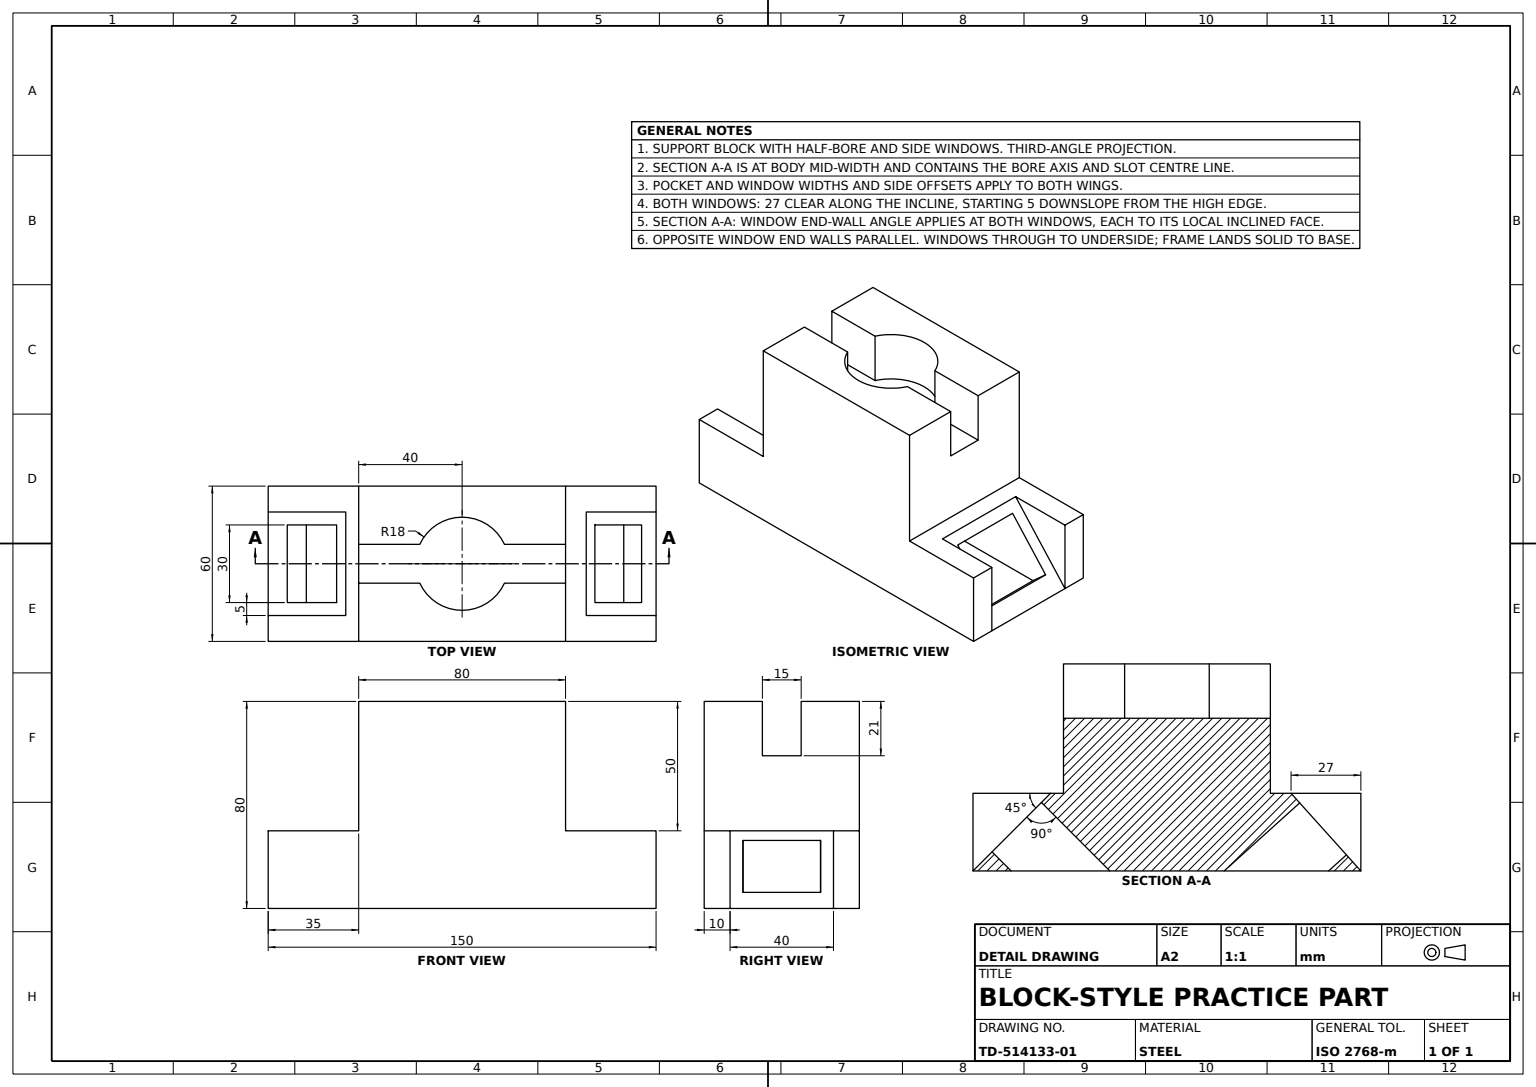
SolidWorks part; units mm, degrees
material "Plain Carbon Steel"
ref_plane "Front Plane" through (0, 0, 0) normal (0, 0, 1) x (1, 0, 0)
ref_plane "Top Plane" through (0, 0, 0) normal (0, 1, 0) x (1, 0, 0)
ref_plane "Right Plane" through (0, 0, 0) normal (1, 0, 0) x (0, 0, -1)
sketch "Base Profile Sketch" plane through (0, 0, 0) normal (0, 0, 1) x (1, 0, 0)
  line L0 (-47.8178, 0) -> (102.1822, 0)
  line L1 (102.1822, 0) -> (102.1822, 30)
  line L2 (102.1822, 30) -> (67.1822, 30)
  line L3 (67.1822, 30) -> (67.1822, 80)
  line L4 (67.1822, 80) -> (-12.8178, 80)
  line L5 (-12.8178, 80) -> (-12.8178, 30)
  line L6 (-12.8178, 30) -> (-47.8178, 30)
  line L7 (-47.8178, 30) -> (-47.8178, 0)
  dimension "D1" = 150
  dimension "D2" = 30
  dimension "D3" = 35
  dimension "D4" = 50
  dimension "D5" = 50
  dimension "D6" = 80
  dimension "D7" = 47.8178
extrude "Base Block" add sketch "Base Profile Sketch" against normal blind 60
sketch "Bore Sketch" plane through (0, 80, 0) normal (0, 1, 0) x (1, 0, 0)
  line L0 (-12.8178, 60) -> (-12.8178, 0) construction
  line L1 (67.1822, 0) -> (-12.8178, 0) construction
  circle A1 centre (27.1822, 30) radius 18
  point P4 (-12.8178, 30)
  dimension "D1" = 18
  dimension "D2" = 40
  dimension "D3" = 30
extrude "Half Bore Cut" cut sketch "Bore Sketch" against normal blind 21
sketch "Top Slot Sketch" plane through (0, 80, 0) normal (0, 1, 0) x (1, 0, 0)
  line L0 (-12.8178, 37.5) -> (-12.8178, 22.5)
  line L1 (67.1822, 37.5) -> (67.1822, 22.5)
  line L3 (-12.8178, 22.5) -> (67.1822, 22.5)
  line L4 (-12.8178, 37.5) -> (67.1822, 37.5)
  dimension "D1" = 15
  dimension "D2" = 80
  dimension "D3" = 12.8178
  dimension "D4" = 22.5
extrude "Top Slot Cut" cut sketch "Top Slot Sketch" against normal blind 21
sketch "Side Pocket A Sketch" plane through (0, 30, 0) normal (0, 1, 0) x (1, 0, 0)
  line L2 (102.1822, 60) -> (102.1822, 0) construction
  line L4 (102.1822, 10) -> (75.1822, 10)
  line L5 (75.1822, 10) -> (75.1822, 50)
  line L6 (75.1822, 50) -> (102.1822, 50)
  line L7 (67.1822, 60) -> (67.1822, 0) construction
  line L8 (102.1822, 50) -> (102.1822, 10)
  line L12 (102.1822, 0) -> (67.1822, 0) construction
  point P10 (88.6822, 10)
  dimension "D1" = 27
  dimension "D2" = 40
  dimension "D3" = 8
  dimension "D4" = 10
extrude "Side Pocket A" cut sketch "Side Pocket A Sketch" against normal blind 40
sketch "Frame Infill A Sketch" plane through (0, 0, -50) normal (0, 0, 1) x (1, 0, 0)
  line L0 (75.1822, 30) -> (102.1822, 0)
  line L1 (102.1822, 0) -> (75.1822, 0)
  line L2 (75.1822, 0) -> (75.1822, 30)
extrude "Frame Infill A" add sketch "Frame Infill A Sketch" along normal blind 40
sketch "Triangle Window A Sketch" plane through (56.4542, 50.8088, 0) normal (0.7433, 0.669, 0) x (0, 0, -1)
  line L0 (50, -27.9954) -> (10, -27.9954) construction
  line L1 (15, -32.9954) -> (45, -32.9954)
  line L2 (15, -32.9954) -> (15, -59.9954)
  line L3 (15, -59.9954) -> (45, -59.9954)
  line L4 (45, -32.9954) -> (45, -59.9954)
  line L5 (15, -32.9954) -> (45, -59.9954) construction
  line L6 (15, -59.9954) -> (45, -32.9954) construction
  line L7 (50, -68.3563) -> (50, -27.9954) construction
  point P0 (30, -46.4954)
  dimension "D1" = 30
  dimension "D2" = 27
  dimension "D3" = 5
  dimension "D4" = 5
extrude "Triangle Window A" cut sketch "Triangle Window A Sketch" against normal blind 40
sketch "Side Pocket B Sketch" plane through (0, 30, 0) normal (0, 1, 0) x (1, 0, 0)
  line L3 (-12.8178, 37.5) -> (-12.8178, 22.5) construction
  line L4 (-47.8178, 50) -> (-17.8178, 50)
  line L5 (-47.8178, 50) -> (-47.8178, 10)
  line L6 (-47.8178, 10) -> (-17.8178, 10)
  line L7 (-17.8178, 50) -> (-17.8178, 10)
  line L8 (-47.8178, 50) -> (-17.8178, 10) construction
  line L9 (-47.8178, 10) -> (-17.8178, 50) construction
  line L10 (-12.8178, 60) -> (-47.8178, 60) construction
  point P6 (-32.8178, 30)
  dimension "D1" = 5
  dimension "D2" = 10
  dimension "D3" = 40
  dimension "D4" = 30
extrude "Side Pocket B" cut sketch "Side Pocket B Sketch" against normal blind 40
sketch "Frame Infill B Sketch" plane through (0, 0, -50) normal (0, 0, 1) x (1, 0, 0)
  line L0 (-47.8178, 0) -> (-17.8178, 30)
  line L1 (-17.8178, 30) -> (-17.8178, 0)
  line L2 (-17.8178, 0) -> (-47.8178, 0)
extrude "Frame Infill B" add sketch "Frame Infill B Sketch" along normal blind 40
sketch "Triangle Window B Sketch" plane through (-23.9089, 23.9089, 0) normal (-0.7071, 0.7071, 0) x (0, 0, 1)
  line L1 (-45, 3.6141) -> (-15, 3.6141)
  line L2 (-45, 3.6141) -> (-45, -23.3859)
  line L3 (-45, -23.3859) -> (-15, -23.3859)
  line L4 (-15, 3.6141) -> (-15, -23.3859)
  line L5 (-45, 3.6141) -> (-15, -23.3859) construction
  line L6 (-45, -23.3859) -> (-15, 3.6141) construction
  line L7 (-50, 8.6141) -> (-50, -33.8123) construction
  line L9 (-10, 8.6141) -> (-50, 8.6141) construction
  point P0 (-30, -9.8859)
  dimension "D1" = 27
  dimension "D2" = 30
  dimension "D3" = 5
  dimension "D4" = 5
extrude "Triangle Window B" cut sketch "Triangle Window B Sketch" against normal blind 40
